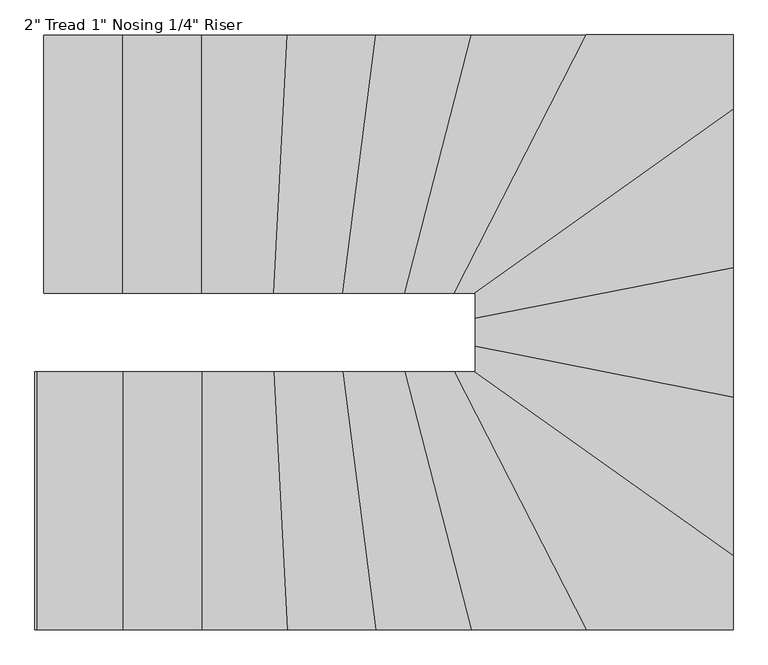
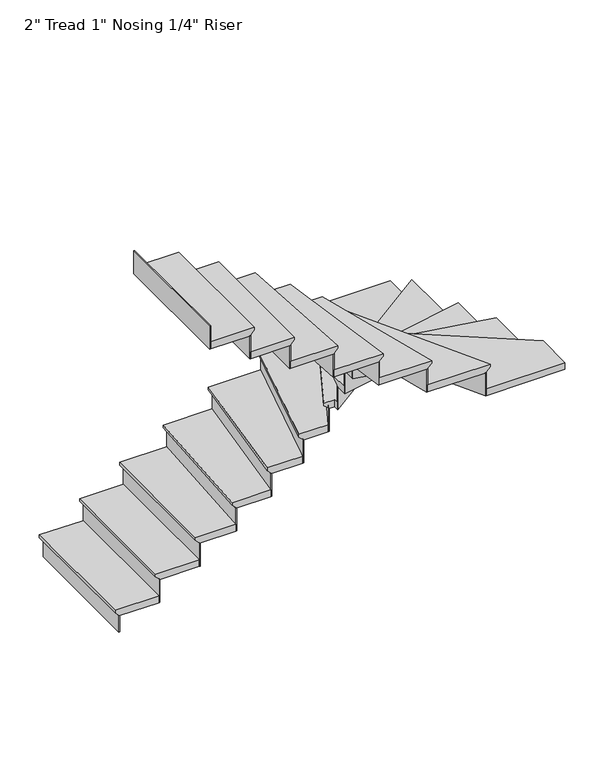
"""IFC4 building model written with IfcOpenShell, lengths in millimetres: stair flight geometry."""

from ifc_helpers import new_model, si_unit, origin, place, context, project, spatial, faceted_brep, source, transform, mapped, element, save


def stair_flight_4d9189d9(model_context):
    return source(origin(), model_context, "Body", "Brep", [
        faceted_brep([(1342.8282136, -2159.7365003, 6551.0833333), (1342.8282136, -2159.7365003, 6570.1333333), (1342.8282136, -1245.3365003, 6570.1333333), (1342.8282136, -1245.3365003, 6551.0833333), (1368.2282136, -2159.7365003, 6525.6833333), (1368.2282136, -1245.3365003, 6525.6833333), (1647.6282136, -2159.7365003, 6570.1333333), (1647.6282136, -1245.3365003, 6570.1333333), (1368.2282136, -1245.3365003, 6519.3333333), (1647.6282136, -1245.3365003, 6519.3333333), (1647.6282136, -2159.7365003, 6519.3333333), (1368.2282136, -2159.7365003, 6519.3333333)], [[[0, 1, 2, 3]], [[4, 0, 3, 5]], [[2, 1, 6, 7]], [[8, 9, 10, 11]], [[2, 7, 9, 8, 5, 3]], [[8, 11, 4, 5]], [[6, 1, 0, 4, 11, 10]], [[7, 6, 10, 9]]]),
        faceted_brep([(1368.2282136, -2159.7365003, 6519.3333333), (1368.2282136, -2159.7365003, 6400.8), (1374.5782136, -2159.7365003, 6400.8), (1374.5782136, -2159.7365003, 6519.3333333), (1368.2282136, -1245.3365003, 6519.3333333), (1374.5782136, -1245.3365003, 6519.3333333), (1374.5782136, -1245.3365003, 6400.8), (1368.2282136, -1245.3365003, 6400.8)], [[[0, 1, 2, 3]], [[4, 5, 6, 7]], [[1, 0, 4, 7]], [[2, 1, 7, 6]], [[3, 2, 6, 5]], [[0, 3, 5, 4]]]),
        faceted_brep([(1647.6282136, -2159.7365003, 6688.6666667), (1647.6282136, -2159.7365003, 6519.3333333), (1653.9782136, -2159.7365003, 6519.3333333), (1653.9782136, -2159.7365003, 6688.6666667), (1647.6282136, -1245.3365003, 6688.6666667), (1653.9782136, -1245.3365003, 6688.6666667), (1653.9782136, -1245.3365003, 6519.3333333), (1647.6282136, -1245.3365003, 6519.3333333)], [[[0, 1, 2, 3]], [[4, 5, 6, 7]], [[1, 0, 4, 7]], [[2, 1, 7, 6]], [[3, 2, 6, 5]], [[0, 3, 5, 4]]]),
        faceted_brep([(1622.2282136, -1245.3365003, 6739.4666667), (1622.2282136, -2159.7365003, 6739.4666667), (1927.0282136, -2159.7365003, 6739.4666667), (1927.0282136, -1245.3365003, 6739.4666667), (1647.6282136, -1245.3365003, 6688.6666667), (1927.0282136, -1245.3365003, 6688.6666667), (1927.0282136, -2159.7365003, 6688.6666667), (1647.6282136, -2159.7365003, 6688.6666667), (1647.6282136, -1245.3365003, 6695.0166667), (1622.2282136, -1245.3365003, 6720.4166667), (1647.6282136, -2159.7365003, 6695.0166667), (1622.2282136, -2159.7365003, 6720.4166667)], [[[0, 1, 2, 3]], [[4, 5, 6, 7]], [[0, 3, 5, 4, 8, 9]], [[4, 7, 10, 8]], [[2, 1, 11, 10, 7, 6]], [[3, 2, 6, 5]], [[11, 1, 0, 9]], [[10, 11, 9, 8]]]),
        faceted_brep([(1927.0282136, -2159.7365003, 6858.0), (1927.0282136, -2159.7365003, 6688.6666667), (1933.3782136, -2159.7365003, 6688.6666667), (1933.3782136, -2159.7365003, 6858.0), (1927.0282136, -1245.3365003, 6858.0), (1933.3782136, -1245.3365003, 6858.0), (1933.3782136, -1245.3365003, 6688.6666667), (1927.0282136, -1245.3365003, 6688.6666667)], [[[0, 1, 2, 3]], [[4, 5, 6, 7]], [[1, 0, 4, 7]], [[2, 1, 7, 6]], [[3, 2, 6, 5]], [[0, 3, 5, 4]]]),
        faceted_brep([(1901.6282136, -1245.3365003, 6908.8), (1901.6282136, -2159.7365003, 6908.8), (2182.6953751, -2159.7365003, 6908.8), (2230.2296455, -1245.3365003, 6908.8), (1927.0282136, -1245.3365003, 6858.0), (2230.2296455, -1245.3365003, 6858.0), (2182.6953751, -2159.7365003, 6858.0), (1927.0282136, -2159.7365003, 6858.0), (1927.0282136, -1245.3365003, 6864.35), (1901.6282136, -1245.3365003, 6889.75), (1927.0282136, -2159.7365003, 6864.35), (1901.6282136, -2159.7365003, 6889.75)], [[[0, 1, 2, 3]], [[4, 5, 6, 7]], [[0, 3, 5, 4, 8, 9]], [[4, 7, 10, 8]], [[2, 1, 11, 10, 7, 6]], [[3, 2, 6, 5]], [[11, 1, 0, 9]], [[10, 11, 9, 8]]]),
        faceted_brep([(2182.6953751, -2159.7365003, 7027.3333333), (2182.6953751, -2159.7365003, 6858.0), (2189.0539493, -2159.7365003, 6858.0), (2189.0539493, -2159.7365003, 7027.3333333), (2230.2296455, -1245.3365003, 7027.3333333), (2236.5882197, -1245.3365003, 7027.3333333), (2236.5882197, -1245.3365003, 6858.0), (2230.2296455, -1245.3365003, 6858.0)], [[[0, 1, 2, 3]], [[4, 5, 6, 7]], [[1, 0, 4, 7]], [[2, 1, 7, 6]], [[3, 2, 6, 5]], [[0, 3, 5, 4]]]),
        faceted_brep([(2204.7953488, -1245.3365003, 7078.1333333), (2157.2610784, -2159.7365003, 7078.1333333), (2426.8620749, -2159.7365003, 7078.1333333), (2545.2181266, -1245.3365003, 7078.1333333), (2230.2296455, -1245.3365003, 7027.3333333), (2545.2181266, -1245.3365003, 7027.3333333), (2426.8620749, -2159.7365003, 7027.3333333), (2182.6953751, -2159.7365003, 7027.3333333), (2230.2296455, -1245.3365003, 7033.6833333), (2204.7953488, -1245.3365003, 7059.0833333), (2182.6953751, -2159.7365003, 7033.6833333), (2157.2610784, -2159.7365003, 7059.0833333)], [[[0, 1, 2, 3]], [[4, 5, 6, 7]], [[0, 3, 5, 4, 8, 9]], [[4, 7, 10, 8]], [[2, 1, 11, 10, 7, 6]], [[3, 2, 6, 5]], [[11, 1, 0, 9]], [[10, 11, 9, 8]]]),
        faceted_brep([(2426.8620749, -2159.7365003, 7196.6666667), (2426.8620749, -2159.7365003, 7027.3333333), (2433.2650467, -2159.7365003, 7027.3333333), (2433.2650467, -2159.7365003, 7196.6666667), (2545.2181266, -1245.3365003, 7196.6666667), (2551.6210984, -1245.3365003, 7196.6666667), (2551.6210984, -1245.3365003, 7027.3333333), (2545.2181266, -1245.3365003, 7027.3333333)], [[[0, 1, 2, 3]], [[4, 5, 6, 7]], [[1, 0, 4, 7]], [[2, 1, 7, 6]], [[3, 2, 6, 5]], [[0, 3, 5, 4]]]),
        faceted_brep([(2519.6062395, -1245.3365003, 7247.4666667), (2401.2501878, -2159.7365003, 7247.4666667), (2648.4892974, -2159.7365003, 7247.4666667), (2883.6197448, -1245.3365003, 7247.4666667), (2545.2181266, -1245.3365003, 7196.6666667), (2883.6197448, -1245.3365003, 7196.6666667), (2648.4892974, -2159.7365003, 7196.6666667), (2426.8620749, -2159.7365003, 7196.6666667), (2545.2181266, -1245.3365003, 7203.0166667), (2519.6062395, -1245.3365003, 7228.4166667), (2426.8620749, -2159.7365003, 7203.0166667), (2401.2501878, -2159.7365003, 7228.4166667)], [[[0, 1, 2, 3]], [[4, 5, 6, 7]], [[0, 3, 5, 4, 8, 9]], [[4, 7, 10, 8]], [[2, 1, 11, 10, 7, 6]], [[3, 2, 6, 5]], [[11, 1, 0, 9]], [[10, 11, 9, 8]]]),
        faceted_brep([(2648.4892974, -2159.7365003, 7366.0), (2648.4892974, -2159.7365003, 7196.6666667), (2655.0458743, -2159.7365003, 7196.6666667), (2655.0458743, -2159.7365003, 7366.0), (2883.6197448, -1245.3365003, 7366.0), (2890.1763217, -1245.3365003, 7366.0), (2890.1763217, -1245.3365003, 7196.6666667), (2883.6197448, -1245.3365003, 7196.6666667)], [[[0, 1, 2, 3]], [[4, 5, 6, 7]], [[1, 0, 4, 7]], [[2, 1, 7, 6]], [[3, 2, 6, 5]], [[0, 3, 5, 4]]]),
        faceted_brep([(2857.3934373, -1245.3365003, 7416.8), (2622.2629899, -2159.7365003, 7416.8), (2824.8359335, -2159.7365003, 7416.8), (3293.6605548, -1245.3365003, 7416.8), (2883.6197448, -1245.3365003, 7366.0), (3293.6605548, -1245.3365003, 7366.0), (2824.8359335, -2159.7365003, 7366.0), (2648.4892974, -2159.7365003, 7366.0), (2883.6197448, -1245.3365003, 7372.35), (2857.3934373, -1245.3365003, 7397.75), (2648.4892974, -2159.7365003, 7372.35), (2622.2629899, -2159.7365003, 7397.75)], [[[0, 1, 2, 3]], [[4, 5, 6, 7]], [[0, 3, 5, 4, 8, 9]], [[4, 7, 10, 8]], [[2, 1, 11, 10, 7, 6]], [[3, 2, 6, 5]], [[11, 1, 0, 9]], [[10, 11, 9, 8]]]),
        faceted_brep([(2824.8359335, -2159.7365003, 7535.3333333), (2824.8359335, -2159.7365003, 7366.0), (2831.9719166, -2159.7365003, 7366.0), (2831.9719166, -2159.7365003, 7535.3333333), (3293.6605548, -1245.3365003, 7535.3333333), (3300.7965379, -1245.3365003, 7535.3333333), (3300.7965379, -1245.3365003, 7366.0), (3293.6605548, -1245.3365003, 7366.0)], [[[0, 1, 2, 3]], [[4, 5, 6, 7]], [[1, 0, 4, 7]], [[2, 1, 7, 6]], [[3, 2, 6, 5]], [[0, 3, 5, 4]]]),
        faceted_brep([(3784.9599055, -1539.017634, 7586.1333333), (3784.9599055, -1245.3365003, 7586.1333333), (3265.1166223, -1245.3365003, 7586.1333333), (2796.2920009, -2159.7365003, 7586.1333333), (2870.5599055, -2159.7365003, 7586.1333333), (2870.5599055, -2189.2915832, 7586.1333333), (3784.9599055, -1245.3365003, 7535.3333333), (3784.9599055, -1539.017634, 7535.3333333), (2870.5599055, -2189.2915832, 7535.3333333), (2870.5599055, -2159.7365003, 7535.3333333), (2824.8359335, -2159.7365003, 7535.3333333), (3293.6605548, -1245.3365003, 7535.3333333), (3293.6605548, -1245.3365003, 7541.6833333), (3265.1166223, -1245.3365003, 7567.0833333), (2824.8359335, -2159.7365003, 7541.6833333), (2796.2920009, -2159.7365003, 7567.0833333)], [[[0, 1, 2, 3, 4, 5]], [[6, 7, 8, 9, 10, 11]], [[1, 0, 7, 6]], [[2, 1, 6, 11, 12, 13]], [[11, 10, 14, 12]], [[4, 3, 15, 14, 10, 9]], [[5, 4, 9, 8]], [[0, 5, 8, 7]], [[15, 3, 2, 13]], [[14, 15, 13, 12]]]),
        faceted_brep([(2870.5599055, -2189.2915832, 7704.6666667), (2870.5599055, -2189.2915832, 7535.3333333), (2870.5599055, -2197.083558, 7535.3333333), (2870.5599055, -2197.083558, 7704.6666667), (3784.9599055, -1539.017634, 7704.6666667), (3784.9599055, -1546.8096088, 7704.6666667), (3784.9599055, -1546.8096088, 7535.3333333), (3784.9599055, -1539.017634, 7535.3333333)], [[[0, 1, 2, 3]], [[4, 5, 6, 7]], [[1, 0, 4, 7]], [[2, 1, 7, 6]], [[3, 2, 6, 5]], [[0, 3, 5, 4]]]),
        faceted_brep([(3784.9599055, -1507.8497349, 7755.4666667), (2870.5599055, -2158.123684, 7755.4666667), (2870.5599055, -2275.7456703, 7755.4666667), (3784.9599055, -2095.5048139, 7755.4666667), (3784.9599055, -1539.017634, 7704.6666667), (3784.9599055, -2095.5048139, 7704.6666667), (2870.5599055, -2275.7456703, 7704.6666667), (2870.5599055, -2189.2915832, 7704.6666667), (3784.9599055, -1539.017634, 7711.0166667), (3784.9599055, -1507.8497349, 7736.4166667), (2870.5599055, -2189.2915832, 7711.0166667), (2870.5599055, -2158.123684, 7736.4166667)], [[[0, 1, 2, 3]], [[4, 5, 6, 7]], [[0, 3, 5, 4, 8, 9]], [[4, 7, 10, 8]], [[2, 1, 11, 10, 7, 6]], [[3, 2, 6, 5]], [[11, 1, 0, 9]], [[10, 11, 9, 8]]]),
        faceted_brep([(2870.5599055, -2275.7456703, 7874.0), (2870.5599055, -2275.7456703, 7704.6666667), (2870.5599055, -2282.2178557, 7704.6666667), (2870.5599055, -2282.2178557, 7874.0), (3784.9599055, -2095.5048139, 7874.0), (3784.9599055, -2101.9769994, 7874.0), (3784.9599055, -2101.9769994, 7704.6666667), (3784.9599055, -2095.5048139, 7704.6666667)], [[[0, 1, 2, 3]], [[4, 5, 6, 7]], [[1, 0, 4, 7]], [[2, 1, 7, 6]], [[3, 2, 6, 5]], [[0, 3, 5, 4]]]),
        faceted_brep([(3784.9599055, -2069.6160722, 7924.8), (2870.5599055, -2249.8569285, 7924.8), (2870.5599055, -2374.9048139, 7924.8), (3784.9599055, -2555.1456703, 7924.8), (3784.9599055, -2095.5048139, 7874.0), (3784.9599055, -2555.1456703, 7874.0), (2870.5599055, -2374.9048139, 7874.0), (2870.5599055, -2275.7456703, 7874.0), (3784.9599055, -2095.5048139, 7880.35), (3784.9599055, -2069.6160722, 7905.75), (2870.5599055, -2275.7456703, 7880.35), (2870.5599055, -2249.8569285, 7905.75)], [[[0, 1, 2, 3]], [[4, 5, 6, 7]], [[0, 3, 5, 4, 8, 9]], [[4, 7, 10, 8]], [[2, 1, 11, 10, 7, 6]], [[3, 2, 6, 5]], [[11, 1, 0, 9]], [[10, 11, 9, 8]]]),
        faceted_brep([(2870.5599055, -2374.9048139, 8043.3333333), (2870.5599055, -2374.9048139, 7874.0), (2870.5599055, -2381.3769994, 7874.0), (2870.5599055, -2381.3769994, 8043.3333333), (3784.9599055, -2555.1456703, 8043.3333333), (3784.9599055, -2561.6178557, 8043.3333333), (3784.9599055, -2561.6178557, 7874.0), (3784.9599055, -2555.1456703, 7874.0)], [[[0, 1, 2, 3]], [[4, 5, 6, 7]], [[1, 0, 4, 7]], [[2, 1, 7, 6]], [[3, 2, 6, 5]], [[0, 3, 5, 4]]]),
        faceted_brep([(3784.9599055, -2529.2569285, 8094.1333333), (2870.5599055, -2349.0160722, 8094.1333333), (2870.5599055, -2439.1365003, 8094.1333333), (2824.464431, -2439.1365003, 8094.1333333), (3784.9599055, -3122.191165, 8094.1333333), (3784.9599055, -2555.1456703, 8043.3333333), (3784.9599055, -3122.191165, 8043.3333333), (2824.464431, -2439.1365003, 8043.3333333), (2870.5599055, -2439.1365003, 8043.3333333), (2870.5599055, -2374.9048139, 8043.3333333), (3784.9599055, -2555.1456703, 8049.6833333), (3784.9599055, -2529.2569285, 8075.0833333), (2870.5599055, -2374.9048139, 8049.6833333), (2870.5599055, -2349.0160722, 8075.0833333)], [[[0, 1, 2, 3, 4]], [[5, 6, 7, 8, 9]], [[0, 4, 6, 5, 10, 11]], [[5, 9, 12, 10]], [[2, 1, 13, 12, 9, 8]], [[3, 2, 8, 7]], [[4, 3, 7, 6]], [[13, 1, 0, 11]], [[12, 13, 11, 10]]]),
        faceted_brep([(2824.464431, -2439.1365003, 8212.6666667), (2824.464431, -2439.1365003, 8043.3333333), (2813.5075385, -2439.1365003, 8043.3333333), (2813.5075385, -2439.1365003, 8212.6666667), (3784.9599055, -3122.191165, 8212.6666667), (3784.9599055, -3129.9831398, 8212.6666667), (3784.9599055, -3129.9831398, 8043.3333333), (3784.9599055, -3122.191165, 8043.3333333)], [[[0, 1, 2, 3]], [[4, 5, 6, 7]], [[1, 0, 4, 7]], [[2, 1, 7, 6]], [[3, 2, 6, 5]], [[0, 3, 5, 4]]]),
        faceted_brep([(3236.5726897, -3353.5365003, 8263.4666667), (3784.9599055, -3353.5365003, 8263.4666667), (3784.9599055, -3091.0232658, 8263.4666667), (2868.2920009, -2439.1365003, 8263.4666667), (2767.7480684, -2439.1365003, 8263.4666667), (3784.9599055, -3353.5365003, 8212.6666667), (3236.5726897, -3353.5365003, 8212.6666667), (2767.7480684, -2439.1365003, 8212.6666667), (2824.464431, -2439.1365003, 8212.6666667), (3784.9599055, -3122.191165, 8212.6666667), (3784.9599055, -3122.191165, 8219.0166667), (3784.9599055, -3091.0232658, 8244.4166667), (2824.464431, -2439.1365003, 8219.0166667), (2868.2920009, -2439.1365003, 8244.4166667)], [[[0, 1, 2, 3, 4]], [[5, 6, 7, 8, 9]], [[1, 0, 6, 5]], [[2, 1, 5, 9, 10, 11]], [[9, 8, 12, 10]], [[4, 3, 13, 12, 8, 7]], [[0, 4, 7, 6]], [[13, 3, 2, 11]], [[12, 13, 11, 10]]]),
        faceted_brep([(2767.7480684, -2439.1365003, 8382.0), (2767.7480684, -2439.1365003, 8212.6666667), (2760.6120853, -2439.1365003, 8212.6666667), (2760.6120853, -2439.1365003, 8382.0), (3236.5726897, -3353.5365003, 8382.0), (3229.4367066, -3353.5365003, 8382.0), (3229.4367066, -3353.5365003, 8212.6666667), (3236.5726897, -3353.5365003, 8212.6666667)], [[[0, 1, 2, 3]], [[4, 5, 6, 7]], [[1, 0, 4, 7]], [[2, 1, 7, 6]], [[3, 2, 6, 5]], [[0, 3, 5, 4]]]),
        faceted_brep([(3265.1166223, -3353.5365003, 8432.8), (2796.2920009, -2439.1365003, 8432.8), (2596.0366825, -2439.1365003, 8432.8), (2831.1671299, -3353.5365003, 8432.8), (3236.5726897, -3353.5365003, 8382.0), (2831.1671299, -3353.5365003, 8382.0), (2596.0366825, -2439.1365003, 8382.0), (2767.7480684, -2439.1365003, 8382.0), (3236.5726897, -3353.5365003, 8388.35), (3265.1166223, -3353.5365003, 8413.75), (2767.7480684, -2439.1365003, 8388.35), (2796.2920009, -2439.1365003, 8413.75)], [[[0, 1, 2, 3]], [[4, 5, 6, 7]], [[0, 3, 5, 4, 8, 9]], [[4, 7, 10, 8]], [[2, 1, 11, 10, 7, 6]], [[3, 2, 6, 5]], [[11, 1, 0, 9]], [[10, 11, 9, 8]]]),
        faceted_brep([(2596.0366825, -2439.1365003, 8551.3333333), (2596.0366825, -2439.1365003, 8382.0), (2589.4801056, -2439.1365003, 8382.0), (2589.4801056, -2439.1365003, 8551.3333333), (2831.1671299, -3353.5365003, 8551.3333333), (2824.610553, -3353.5365003, 8551.3333333), (2824.610553, -3353.5365003, 8382.0), (2831.1671299, -3353.5365003, 8382.0)], [[[0, 1, 2, 3]], [[4, 5, 6, 7]], [[1, 0, 4, 7]], [[2, 1, 7, 6]], [[3, 2, 6, 5]], [[0, 3, 5, 4]]]),
        faceted_brep([(2857.3934373, -3353.5365003, 8602.1333333), (2622.2629899, -2439.1365003, 8602.1333333), (2375.6383007, -2439.1365003, 8602.1333333), (2493.9943524, -3353.5365003, 8602.1333333), (2831.1671299, -3353.5365003, 8551.3333333), (2493.9943524, -3353.5365003, 8551.3333333), (2375.6383007, -2439.1365003, 8551.3333333), (2596.0366825, -2439.1365003, 8551.3333333), (2831.1671299, -3353.5365003, 8557.6833333), (2857.3934373, -3353.5365003, 8583.0833333), (2596.0366825, -2439.1365003, 8557.6833333), (2622.2629899, -2439.1365003, 8583.0833333)], [[[0, 1, 2, 3]], [[4, 5, 6, 7]], [[0, 3, 5, 4, 8, 9]], [[4, 7, 10, 8]], [[2, 1, 11, 10, 7, 6]], [[3, 2, 6, 5]], [[11, 1, 0, 9]], [[10, 11, 9, 8]]]),
        faceted_brep([(2375.6383007, -2439.1365003, 8720.6666667), (2375.6383007, -2439.1365003, 8551.3333333), (2369.2353289, -2439.1365003, 8551.3333333), (2369.2353289, -2439.1365003, 8720.6666667), (2493.9943524, -3353.5365003, 8720.6666667), (2487.5913806, -3353.5365003, 8720.6666667), (2487.5913806, -3353.5365003, 8551.3333333), (2493.9943524, -3353.5365003, 8551.3333333)], [[[0, 1, 2, 3]], [[4, 5, 6, 7]], [[1, 0, 4, 7]], [[2, 1, 7, 6]], [[3, 2, 6, 5]], [[0, 3, 5, 4]]]),
        faceted_brep([(2519.6062395, -3353.5365003, 8771.4666667), (2401.2501878, -2439.1365003, 8771.4666667), (2131.8267818, -2439.1365003, 8771.4666667), (2179.3610522, -3353.5365003, 8771.4666667), (2493.9943524, -3353.5365003, 8720.6666667), (2179.3610522, -3353.5365003, 8720.6666667), (2131.8267818, -2439.1365003, 8720.6666667), (2375.6383007, -2439.1365003, 8720.6666667), (2493.9943524, -3353.5365003, 8727.0166667), (2519.6062395, -3353.5365003, 8752.4166667), (2375.6383007, -2439.1365003, 8727.0166667), (2401.2501878, -2439.1365003, 8752.4166667)], [[[0, 1, 2, 3]], [[4, 5, 6, 7]], [[0, 3, 5, 4, 8, 9]], [[4, 7, 10, 8]], [[2, 1, 11, 10, 7, 6]], [[3, 2, 6, 5]], [[11, 1, 0, 9]], [[10, 11, 9, 8]]]),
        faceted_brep([(2131.8267818, -2439.1365003, 8890.0), (2131.8267818, -2439.1365003, 8720.6666667), (2125.4682076, -2439.1365003, 8720.6666667), (2125.4682076, -2439.1365003, 8890.0), (2179.3610522, -3353.5365003, 8890.0), (2173.002478, -3353.5365003, 8890.0), (2173.002478, -3353.5365003, 8720.6666667), (2179.3610522, -3353.5365003, 8720.6666667)], [[[0, 1, 2, 3]], [[4, 5, 6, 7]], [[1, 0, 4, 7]], [[2, 1, 7, 6]], [[3, 2, 6, 5]], [[0, 3, 5, 4]]]),
        faceted_brep([(2204.7953488, -3353.5365003, 8940.8), (2157.2610784, -2439.1365003, 8940.8), (1876.2282136, -2439.1365003, 8940.8), (1876.2282136, -3353.5365003, 8940.8), (2179.3610522, -3353.5365003, 8890.0), (1876.2282136, -3353.5365003, 8890.0), (1876.2282136, -2439.1365003, 8890.0), (2131.8267818, -2439.1365003, 8890.0), (2179.3610522, -3353.5365003, 8896.35), (2204.7953488, -3353.5365003, 8921.75), (2131.8267818, -2439.1365003, 8896.35), (2157.2610784, -2439.1365003, 8921.75)], [[[0, 1, 2, 3]], [[4, 5, 6, 7]], [[0, 3, 5, 4, 8, 9]], [[4, 7, 10, 8]], [[2, 1, 11, 10, 7, 6]], [[3, 2, 6, 5]], [[11, 1, 0, 9]], [[10, 11, 9, 8]]]),
        faceted_brep([(1876.2282136, -2439.1365003, 9059.3333333), (1876.2282136, -2439.1365003, 8890.0), (1869.8782136, -2439.1365003, 8890.0), (1869.8782136, -2439.1365003, 9059.3333333), (1876.2282136, -3353.5365003, 9059.3333333), (1869.8782136, -3353.5365003, 9059.3333333), (1869.8782136, -3353.5365003, 8890.0), (1876.2282136, -3353.5365003, 8890.0)], [[[0, 1, 2, 3]], [[4, 5, 6, 7]], [[1, 0, 4, 7]], [[2, 1, 7, 6]], [[3, 2, 6, 5]], [[0, 3, 5, 4]]]),
        faceted_brep([(1901.6282136, -3353.5365003, 9110.1333333), (1901.6282136, -2439.1365003, 9110.1333333), (1596.8282136, -2439.1365003, 9110.1333333), (1596.8282136, -3353.5365003, 9110.1333333), (1876.2282136, -3353.5365003, 9059.3333333), (1596.8282136, -3353.5365003, 9059.3333333), (1596.8282136, -2439.1365003, 9059.3333333), (1876.2282136, -2439.1365003, 9059.3333333), (1876.2282136, -3353.5365003, 9065.6833333), (1901.6282136, -3353.5365003, 9091.0833333), (1876.2282136, -2439.1365003, 9065.6833333), (1901.6282136, -2439.1365003, 9091.0833333)], [[[0, 1, 2, 3]], [[4, 5, 6, 7]], [[0, 3, 5, 4, 8, 9]], [[4, 7, 10, 8]], [[2, 1, 11, 10, 7, 6]], [[3, 2, 6, 5]], [[11, 1, 0, 9]], [[10, 11, 9, 8]]]),
        faceted_brep([(1596.8282136, -2439.1365003, 9228.6666667), (1596.8282136, -2439.1365003, 9059.3333333), (1590.4782136, -2439.1365003, 9059.3333333), (1590.4782136, -2439.1365003, 9228.6666667), (1596.8282136, -3353.5365003, 9228.6666667), (1590.4782136, -3353.5365003, 9228.6666667), (1590.4782136, -3353.5365003, 9059.3333333), (1596.8282136, -3353.5365003, 9059.3333333)], [[[0, 1, 2, 3]], [[4, 5, 6, 7]], [[1, 0, 4, 7]], [[2, 1, 7, 6]], [[3, 2, 6, 5]], [[0, 3, 5, 4]]]),
        faceted_brep([(1317.4282136, -2439.1365003, 9398.0), (1317.4282136, -2439.1365003, 9228.6666667), (1311.0782136, -2439.1365003, 9228.6666667), (1311.0782136, -2439.1365003, 9398.0), (1317.4282136, -3353.5365003, 9398.0), (1311.0782136, -3353.5365003, 9398.0), (1311.0782136, -3353.5365003, 9228.6666667), (1317.4282136, -3353.5365003, 9228.6666667)], [[[0, 1, 2, 3]], [[4, 5, 6, 7]], [[1, 0, 4, 7]], [[2, 1, 7, 6]], [[3, 2, 6, 5]], [[0, 3, 5, 4]]]),
        faceted_brep([(1622.2282136, -3353.5365003, 9279.4666667), (1622.2282136, -2439.1365003, 9279.4666667), (1317.4282136, -2439.1365003, 9279.4666667), (1317.4282136, -3353.5365003, 9279.4666667), (1596.8282136, -3353.5365003, 9228.6666667), (1317.4282136, -3353.5365003, 9228.6666667), (1317.4282136, -2439.1365003, 9228.6666667), (1596.8282136, -2439.1365003, 9228.6666667), (1596.8282136, -3353.5365003, 9235.0166667), (1622.2282136, -3353.5365003, 9260.4166667), (1596.8282136, -2439.1365003, 9235.0166667), (1622.2282136, -2439.1365003, 9260.4166667)], [[[0, 1, 2, 3]], [[4, 5, 6, 7]], [[0, 3, 5, 4, 8, 9]], [[4, 7, 10, 8]], [[2, 1, 11, 10, 7, 6]], [[3, 2, 6, 5]], [[11, 1, 0, 9]], [[10, 11, 9, 8]]]),
    ])


if __name__ == "__main__":
    model = new_model("IFC4")
    model_context = context("Model", 3, world=origin())
    ifc_project = project(units=[si_unit("LENGTHUNIT", "METRE", prefix="MILLI")], contexts=[model_context])
    site = spatial("IfcSite", under=ifc_project)
    building = spatial("IfcBuilding", under=site)
    placement = place(None, origin())
    stair_flight_shape = stair_flight_4d9189d9(model_context)
    element("IfcStairFlight", 1, ObjectType="2\" Tread 1\" Nosing 1/4\" Riser", at=placement, inside=building, context=model_context, shape_type="MappedRepresentation", body=[
        mapped(stair_flight_shape, transform((0.0, 0.0, 0.0), x_axis=(1.0, 0.0, 0.0), y_axis=(0.0, 1.0, 0.0), z_axis=(0.0, 0.0, 1.0))),
    ])
    save(model, "model.ifc")
